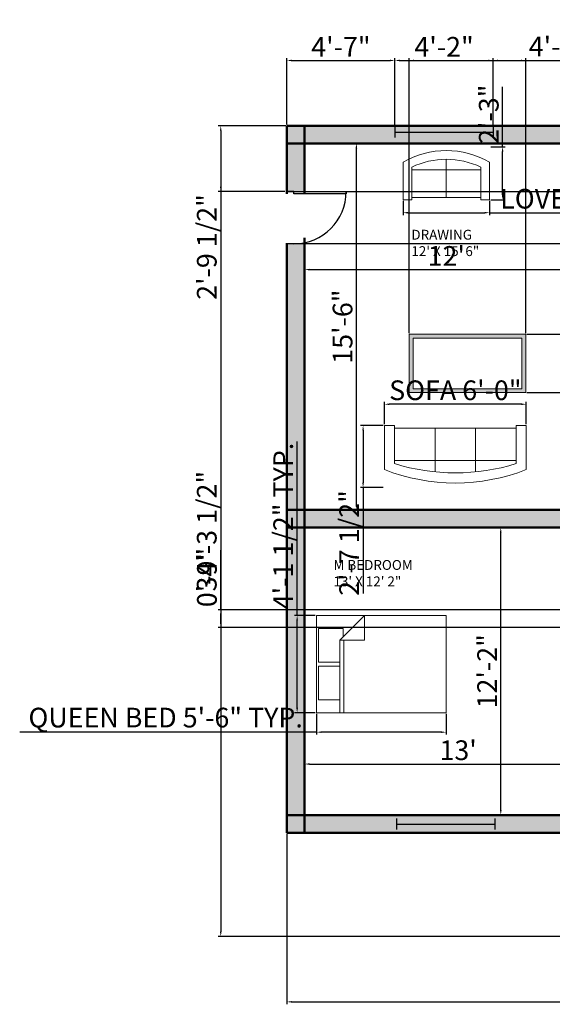
# Model space of a CAD drawing. Units: millimetres. Extents: x 2208 to 3043, y 878 to 1386.
# Tile 1 of 4: x 2208 to 2479, y 886 to 1386. Entities that reach past the tile are written whole.
import ezdxf

# ---------------------------------------------------------------- set-up
doc = ezdxf.new("R2010")
doc.units = ezdxf.units.MM
for name, color, linetype, lineweight in [('A-ANNO-DIMS', 50, 'Continuous', 13), ('A-AREA-IDEN', 90, 'Continuous', 25), ('A-WALL-PATT', 6, 'Continuous', 13), ('doors', 30, 'Continuous', 25), ('furniture', 140, 'Continuous', 18), ('walls', 200, 'Continuous', 50), ('windows', 10, 'Continuous', 25)]:
    doc.layers.add(name, color=color, linetype=linetype, lineweight=lineweight)
doc.layers.add('A-FURN-PATT', color=152, linetype='Continuous', lineweight=13, true_color=0x2776bb)
doc.styles.get("Standard").update_dxf_attribs({"font": 'arial.ttf'})
doc.dimstyles.new('ISO-25', dxfattribs={"dimtxt": 10, "dimasz": 2.5, "dimexe": 1.25, "dimexo": 0.625, "dimtad": 1, "dimdec": 0, "dimlunit": 3, "dimtxsty": 'Standard', "dimcen": 2.5, "dimadec": 0, "dimazin": 0, "dimtfac": 1, "dimtdec": 0, "dimtmove": 0, "dimatfit": 3, "dimfxl": 1, "dimarcsym": 0})

# ---------------------------------------------------------------- blocks, each defined once
blk = doc.blocks.new('*U2')
for p, q in [((0, 0), (0, -6)), ((40, 0), (40, -6))]:
    blk.add_line(p, q)
blk.add_lwpolyline([(0, 0), (0, 40), (1.75, 40), (1.75, 0)], close=True)
blk.add_arc((0, 0), 40, 0, 90)
blk = doc.blocks.new('*U4')
for p, q in [((0, 4), (0, 0)), ((36, 4), (36, 0)), ((0, 2), (36, 2))]:
    blk.add_line(p, q)
blk = doc.blocks.new('Bed - Queen')
for p, q in [((0, -80.00003), (0, 0)), ((0, 0), (59.99999, 0)), ((59.99999, 0), (59.99999, -80.00003)), ((7.99999, -1.2), (28.79998, -1.2)), ((7.99999, -14.4), (7.99999, -1.2)), ((28.79998, -1.2), (28.79998, -14.4)), ((31.19999, -1.2), (51.99999, -1.2)), ((31.19999, -14.4), (31.19999, -1.2)), ((51.99999, -1.2), (51.99999, -16.4)), ((0, -14.4), (44.8, -14.4)), ((44.8, -16.8), (0, -16.8)), ((59.99999, -29.6), (44.8, -14.4)), ((44.8, -14.4), (44.8, -29.6)), ((51.99999, -16.4), (46.79936, -16.4)), ((44.8, -29.6), (59.99999, -29.6)), ((59.99999, -80.00003), (0, -80.00003))]:
    blk.add_line(p, q)
blk = doc.blocks.new('Sofa - Roundback 7 ft.')
for p, q in [((-36.000027, -34), (-36.000027, -11.4696)), ((-12.00002, -32.4421), (-12.00003, -6.5971)), ((11.99997, -32.4421), (11.99998, -6.5971)), ((35.99998, -34), (35.99998, -11.4696)), ((-35.999844, -13.3819), (35.9998, -13.3819)), ((-36.000027, -32.4421), (35.99998, -32.4421))]:
    blk.add_line(p, q)
for points in [[(-36.000027, -34), (-42.000027, -34), (-42.000027, -8)], [(41.99998, -8), (41.99998, -34), (35.99998, -34)]]:
    blk.add_lwpolyline(points)
for centre, radius, start, end in [((0, -114.25), 114.25, 68.43141, 111.5686), ((-0.00001, -127.1968), 121.1968, 72.72033, 107.2797)]:
    blk.add_arc(centre, radius, start, end)
blk = doc.blocks.new('Sofa - Roundback Loveseat 5 ft.')
for p, q in [((0, -32.44198), (0, -5.99998)), ((-24, -33.99998), (-24, -11.46958)), ((-23.9998, -13.38178), (23.99986, -13.38178)), ((24.00004, -33.99998), (24.00004, -11.46958)), ((-24, -32.44198), (24.00004, -32.44198))]:
    blk.add_line(p, q)
for points in [[(-24, -33.99998), (-30, -33.99998), (-30, -7.99998)], [(30.00004, -7.99998), (30.00004, -33.99998), (24.00004, -33.99998)]]:
    blk.add_lwpolyline(points)
for centre, radius, start, end in [((0, -60.24998), 60.24998, 60.13715, 119.8628), ((0, -61.38438), 55.38444, 64.32083, 115.6792)]:
    blk.add_arc(centre, radius, start, end)
blk = doc.blocks.new('*D15')
at = {"layer": 'A-ANNO-DIMS', "color": 0, "lineweight": -2, "transparency": 16777216}
for p, q in [((2352.98, 1251.32), (2352.98, 1260.64)), ((2496.98, 1251.32), (2496.98, 1260.64)), ((2355.48, 1259.39), (2494.48, 1259.39))]:
    blk.add_line(p, q, dxfattribs=at)
at = {"layer": 'A-ANNO-DIMS', "color": 0, "transparency": 16777216}
for points in [[(2355.48, 1259.81), (2355.48, 1258.97), (2352.98, 1259.39)], [(2494.48, 1259.81), (2494.48, 1258.97), (2496.98, 1259.39)]]:
    blk.add_solid(points, dxfattribs=at)
at = {"layer": 'Defpoints', "color": 0, "transparency": 16777216}
for p in [(2496.98, 1259.39), (2352.98, 1250.7), (2496.98, 1250.7)]:
    blk.add_point(p, dxfattribs=at)
at = {"layer": 'A-ANNO-DIMS', "color": 0, "transparency": 16777216, "insert": (2424.98, 1265.03), "char_height": 10, "attachment_point": 5}
blk.add_mtext("12'", dxfattribs=at)
blk = doc.blocks.new('*D16')
at = {"layer": 'A-ANNO-DIMS', "color": 0, "lineweight": -2, "transparency": 16777216}
for p, q in [((2376.11, 1323.44), (2380.54, 1323.44)), ((2379.29, 1139.94), (2379.29, 1320.94)), ((2372.31, 1137.44), (2380.54, 1137.44))]:
    blk.add_line(p, q, dxfattribs=at)
at = {"layer": 'A-ANNO-DIMS', "color": 0, "transparency": 16777216}
for points in [[(2378.87, 1320.94), (2379.71, 1320.94), (2379.29, 1323.44)], [(2378.87, 1139.94), (2379.71, 1139.94), (2379.29, 1137.44)]]:
    blk.add_solid(points, dxfattribs=at)
at = {"layer": 'Defpoints', "color": 0, "transparency": 16777216}
for p in [(2375.49, 1323.44), (2379.29, 1323.44), (2371.69, 1137.44)]:
    blk.add_point(p, dxfattribs=at)
at = {"layer": 'A-ANNO-DIMS', "color": 0, "transparency": 16777216, "insert": (2373.56, 1230.44), "char_height": 10, "attachment_point": 5, "rotation": 90}
blk.add_mtext('15\'-6"', dxfattribs=at)
blk = doc.blocks.new('*D21')
at = {"layer": 'A-ANNO-DIMS', "color": 0, "lineweight": -2, "transparency": 16777216}
for p, q in [((2470.86, 1128.44), (2451.4, 1128.44)), ((2452.65, 984.94), (2452.65, 1125.94)), ((2470.86, 982.44), (2451.4, 982.44))]:
    blk.add_line(p, q, dxfattribs=at)
at = {"layer": 'A-ANNO-DIMS', "color": 0, "transparency": 16777216}
for points in [[(2452.23, 1125.94), (2453.07, 1125.94), (2452.65, 1128.44)], [(2452.23, 984.94), (2453.07, 984.94), (2452.65, 982.44)]]:
    blk.add_solid(points, dxfattribs=at)
at = {"layer": 'Defpoints', "color": 0, "transparency": 16777216}
for p in [(2452.65, 1128.44), (2471.48, 1128.44), (2471.48, 982.44)]:
    blk.add_point(p, dxfattribs=at)
at = {"layer": 'A-ANNO-DIMS', "color": 0, "transparency": 16777216, "insert": (2447, 1055.44), "char_height": 10, "attachment_point": 5, "rotation": 90}
blk.add_mtext('12\'-2"', dxfattribs=at)
blk = doc.blocks.new('*D22')
at = {"layer": 'A-ANNO-DIMS', "color": 0, "lineweight": -2, "transparency": 16777216}
for p, q in [((2352.98, 996.86), (2352.98, 1009.56)), ((2355.48, 1008.31), (2506.48, 1008.31)), ((2508.98, 996.86), (2508.98, 1009.56))]:
    blk.add_line(p, q, dxfattribs=at)
at = {"layer": 'A-ANNO-DIMS', "color": 0, "transparency": 16777216}
for points in [[(2355.48, 1008.73), (2355.48, 1007.9), (2352.98, 1008.31)], [(2506.48, 1008.73), (2506.48, 1007.9), (2508.98, 1008.31)]]:
    blk.add_solid(points, dxfattribs=at)
at = {"layer": 'Defpoints', "color": 0, "transparency": 16777216}
for p in [(2508.98, 1008.31), (2352.98, 996.23), (2508.98, 996.23)]:
    blk.add_point(p, dxfattribs=at)
at = {"layer": 'A-ANNO-DIMS', "color": 0, "transparency": 16777216, "insert": (2430.98, 1014.05), "char_height": 10, "attachment_point": 5}
blk.add_mtext("13'", dxfattribs=at)
blk = doc.blocks.new('*D36')
at = {"layer": 'A-ANNO-DIMS', "color": 0, "lineweight": -2, "transparency": 16777216}
for p, q in [((2359.06, 1033.76), (2359.06, 1023.26)), ((2424.9, 1033.76), (2424.9, 1023.26)), ((2359.06, 1024.51), (2208.21, 1024.51)), ((2422.4, 1024.51), (2361.56, 1024.51))]:
    blk.add_line(p, q, dxfattribs=at)
at = {"layer": 'A-ANNO-DIMS', "color": 0, "transparency": 16777216}
for points in [[(2361.56, 1024.92), (2361.56, 1024.09), (2359.06, 1024.51)], [(2422.4, 1024.92), (2422.4, 1024.09), (2424.9, 1024.51)]]:
    blk.add_solid(points, dxfattribs=at)
at = {"layer": 'Defpoints', "color": 0, "transparency": 16777216}
for p in [(2359.06, 1034.38), (2424.9, 1034.38), (2359.06, 1024.51)]:
    blk.add_point(p, dxfattribs=at)
at = {"layer": 'A-ANNO-DIMS', "color": 0, "transparency": 16777216, "insert": (2282.38, 1030.61), "char_height": 10, "attachment_point": 5}
blk.add_mtext('QUEEN BED 5\'-6" TYP.', dxfattribs=at)
blk = doc.blocks.new('*D37')
at = {"layer": 'A-ANNO-DIMS', "color": 0, "lineweight": -2, "transparency": 16777216}
for p, q in [((2349.18, 1083.76), (2349.18, 1172.17)), ((2358.43, 1083.76), (2347.93, 1083.76)), ((2349.18, 1036.88), (2349.18, 1081.26)), ((2358.43, 1034.38), (2347.93, 1034.38))]:
    blk.add_line(p, q, dxfattribs=at)
at = {"layer": 'A-ANNO-DIMS', "color": 0, "transparency": 16777216}
for points in [[(2348.77, 1081.26), (2349.6, 1081.26), (2349.18, 1083.76)], [(2348.77, 1036.88), (2349.6, 1036.88), (2349.18, 1034.38)]]:
    blk.add_solid(points, dxfattribs=at)
at = {"layer": 'Defpoints', "color": 0, "transparency": 16777216}
for p in [(2349.18, 1083.76), (2359.06, 1083.76), (2359.06, 1034.38)]:
    blk.add_point(p, dxfattribs=at)
at = {"layer": 'A-ANNO-DIMS', "color": 0, "transparency": 16777216, "insert": (2343.39, 1129.22), "char_height": 10, "attachment_point": 5, "rotation": 90}
blk.add_mtext('4\'-1 1/2" TYP.', dxfattribs=at)
blk = doc.blocks.new('*D42')
at = {"layer": 'A-ANNO-DIMS', "color": 0, "lineweight": -2, "transparency": 16777216}
for p, q in [((2393.52, 1180.83), (2393.52, 1192.27)), ((2463.14, 1191.02), (2396.02, 1191.02)), ((2465.64, 1180.83), (2465.64, 1192.27))]:
    blk.add_line(p, q, dxfattribs=at)
at = {"layer": 'A-ANNO-DIMS', "color": 0, "transparency": 16777216}
for points in [[(2396.02, 1191.44), (2396.02, 1190.61), (2393.52, 1191.02)], [(2463.14, 1191.44), (2463.14, 1190.61), (2465.64, 1191.02)]]:
    blk.add_solid(points, dxfattribs=at)
at = {"layer": 'Defpoints', "color": 0, "transparency": 16777216}
for p in [(2393.52, 1191.02), (2393.52, 1180.2), (2465.64, 1180.2)]:
    blk.add_point(p, dxfattribs=at)
at = {"layer": 'A-ANNO-DIMS', "color": 0, "transparency": 16777216, "insert": (2429.58, 1196.82), "char_height": 10, "attachment_point": 5}
blk.add_mtext('SOFA 6\'-0"', dxfattribs=at)
blk = doc.blocks.new('*D43')
at = {"layer": 'A-ANNO-DIMS', "color": 0, "lineweight": -2, "transparency": 16777216}
for p, q in [((2392.89, 1180.2), (2381.45, 1180.2)), ((2382.7, 1177.7), (2382.7, 1151.22)), ((2392.89, 1148.72), (2381.45, 1148.72)), ((2382.7, 1148.72), (2382.7, 1094.92))]:
    blk.add_line(p, q, dxfattribs=at)
at = {"layer": 'A-ANNO-DIMS', "color": 0, "transparency": 16777216}
for points in [[(2382.29, 1177.7), (2383.12, 1177.7), (2382.7, 1180.2)], [(2382.29, 1151.22), (2383.12, 1151.22), (2382.7, 1148.72)]]:
    blk.add_solid(points, dxfattribs=at)
at = {"layer": 'Defpoints', "color": 0, "transparency": 16777216}
for p in [(2393.52, 1180.2), (2382.7, 1148.72), (2393.52, 1148.72)]:
    blk.add_point(p, dxfattribs=at)
at = {"layer": 'A-ANNO-DIMS', "color": 0, "transparency": 16777216, "insert": (2376.91, 1120.57), "char_height": 10, "attachment_point": 5, "rotation": 90}
blk.add_mtext('2\'-7 1/2"', dxfattribs=at)
blk = doc.blocks.new('*D44')
at = {"layer": 'A-ANNO-DIMS', "color": 0, "lineweight": -2, "transparency": 16777216}
for p, q in [((2402.99, 1294.26), (2402.99, 1287.04)), ((2446.98, 1294.26), (2446.98, 1287.04)), ((2405.49, 1288.29), (2444.48, 1288.29)), ((2446.98, 1288.29), (2554.51, 1288.29))]:
    blk.add_line(p, q, dxfattribs=at)
at = {"layer": 'A-ANNO-DIMS', "color": 0, "transparency": 16777216}
for points in [[(2405.49, 1288.7), (2405.49, 1287.87), (2402.99, 1288.29)], [(2444.48, 1288.7), (2444.48, 1287.87), (2446.98, 1288.29)]]:
    blk.add_solid(points, dxfattribs=at)
at = {"layer": 'Defpoints', "color": 0, "transparency": 16777216}
for p in [(2402.99, 1294.89), (2446.98, 1294.89), (2446.98, 1288.29)]:
    blk.add_point(p, dxfattribs=at)
at = {"layer": 'A-ANNO-DIMS', "color": 0, "transparency": 16777216, "insert": (2502, 1294.09), "char_height": 10, "attachment_point": 5}
blk.add_mtext('LOVESEAT 3\'-8"', dxfattribs=at)
blk = doc.blocks.new('*D45')
at = {"layer": 'A-ANNO-DIMS', "color": 0, "lineweight": -2, "transparency": 16777216}
for p, q in [((2453.58, 1321.77), (2453.58, 1352.28)), ((2447.61, 1321.77), (2454.83, 1321.77)), ((2453.58, 1297.39), (2453.58, 1319.27)), ((2447.61, 1294.89), (2454.83, 1294.89))]:
    blk.add_line(p, q, dxfattribs=at)
at = {"layer": 'A-ANNO-DIMS', "color": 0, "transparency": 16777216}
for points in [[(2453.17, 1319.27), (2454, 1319.27), (2453.58, 1321.77)], [(2453.17, 1297.39), (2454, 1297.39), (2453.58, 1294.89)]]:
    blk.add_solid(points, dxfattribs=at)
at = {"layer": 'Defpoints', "color": 0, "transparency": 16777216}
for p in [(2446.98, 1321.77), (2453.58, 1321.77), (2446.98, 1294.89)]:
    blk.add_point(p, dxfattribs=at)
at = {"layer": 'A-ANNO-DIMS', "color": 0, "transparency": 16777216, "insert": (2447.85, 1338.28), "char_height": 10, "attachment_point": 5, "rotation": 90}
blk.add_mtext('2\'-3"', dxfattribs=at)
blk = doc.blocks.new('*D46')
at = {"layer": 'A-ANNO-DIMS', "color": 0, "lineweight": -2, "transparency": 16777216}
for p, q in [((3001.16, 1077), (3001.16, 886.32)), ((2343.98, 972.81), (2343.98, 886.32)), ((2346.48, 887.57), (2998.66, 887.57))]:
    blk.add_line(p, q, dxfattribs=at)
at = {"layer": 'A-ANNO-DIMS', "color": 0, "transparency": 16777216}
for points in [[(2346.48, 887.99), (2346.48, 887.16), (2343.98, 887.57)], [(2998.66, 887.99), (2998.66, 887.16), (3001.16, 887.57)]]:
    blk.add_solid(points, dxfattribs=at)
at = {"layer": 'Defpoints', "color": 0, "transparency": 16777216}
for p in [(3001.16, 1077.62), (2343.98, 973.44), (3001.16, 887.57)]:
    blk.add_point(p, dxfattribs=at)
at = {"layer": 'A-ANNO-DIMS', "color": 0, "transparency": 16777216, "insert": (2672.57, 893.3), "char_height": 10, "attachment_point": 5}
blk.add_mtext('54\'-9"', dxfattribs=at)
blk = doc.blocks.new('*D47')
at = {"layer": 'A-ANNO-DIMS', "color": 0, "lineweight": -2, "transparency": 16777216}
for p, q in [((2343.36, 1332.44), (2309.12, 1332.44)), ((2310.37, 1329.94), (2310.37, 923.22)), ((2589.36, 920.72), (2309.12, 920.72))]:
    blk.add_line(p, q, dxfattribs=at)
at = {"layer": 'A-ANNO-DIMS', "color": 0, "transparency": 16777216}
for points in [[(2309.95, 1329.94), (2310.79, 1329.94), (2310.37, 1332.44)], [(2309.95, 923.22), (2310.79, 923.22), (2310.37, 920.72)]]:
    blk.add_solid(points, dxfattribs=at)
at = {"layer": 'Defpoints', "color": 0, "transparency": 16777216}
for p in [(2343.98, 1332.44), (2310.37, 920.72), (2589.98, 920.72)]:
    blk.add_point(p, dxfattribs=at)
at = {"layer": 'A-ANNO-DIMS', "color": 0, "transparency": 16777216, "insert": (2304.57, 1126.58), "char_height": 10, "attachment_point": 5, "rotation": 90}
blk.add_mtext('34\'-3 1/2"', dxfattribs=at)
blk = doc.blocks.new('*D51')
at = {"layer": 'A-ANNO-DIMS', "color": 0, "lineweight": -2, "transparency": 16777216}
for p, q in [((2344.15, 1299.03), (3035.56, 1299.03)), ((3034.31, 1296.53), (3034.31, 1275.14)), ((2344.61, 1272.64), (3035.56, 1272.64)), ((3034.31, 1272.64), (3034.31, 1218.83))]:
    blk.add_line(p, q, dxfattribs=at)
at = {"layer": 'A-ANNO-DIMS', "color": 0, "transparency": 16777216}
for points in [[(3033.9, 1296.53), (3034.73, 1296.53), (3034.31, 1299.03)], [(3033.9, 1275.14), (3034.73, 1275.14), (3034.31, 1272.64)]]:
    blk.add_solid(points, dxfattribs=at)
at = {"layer": 'Defpoints', "color": 0, "transparency": 16777216}
for p in [(2343.52, 1299.03), (2343.98, 1272.64), (3034.31, 1272.64)]:
    blk.add_point(p, dxfattribs=at)
at = {"layer": 'A-ANNO-DIMS', "color": 0, "transparency": 16777216, "insert": (3028.52, 1244.49), "char_height": 10, "attachment_point": 5, "rotation": 90}
blk.add_mtext('2\'-2 1/2"', dxfattribs=at)
blk = doc.blocks.new('*D52')
at = {"layer": 'A-ANNO-DIMS', "color": 0, "lineweight": -2, "transparency": 16777216}
for p, q in [((2343.36, 1332.44), (2309.12, 1332.44)), ((2310.37, 1329.94), (2310.37, 1301.53)), ((2342.9, 1299.03), (2309.12, 1299.03)), ((2310.37, 1299.03), (2310.37, 1245.23))]:
    blk.add_line(p, q, dxfattribs=at)
at = {"layer": 'A-ANNO-DIMS', "color": 0, "transparency": 16777216}
for points in [[(2309.95, 1329.94), (2310.79, 1329.94), (2310.37, 1332.44)], [(2309.95, 1301.53), (2310.79, 1301.53), (2310.37, 1299.03)]]:
    blk.add_solid(points, dxfattribs=at)
at = {"layer": 'Defpoints', "color": 0, "transparency": 16777216}
for p in [(2343.98, 1332.44), (2310.37, 1299.03), (2343.52, 1299.03)]:
    blk.add_point(p, dxfattribs=at)
at = {"layer": 'A-ANNO-DIMS', "color": 0, "transparency": 16777216, "insert": (2304.57, 1270.88), "char_height": 10, "attachment_point": 5, "rotation": 90}
blk.add_mtext('2\'-9 1/2"', dxfattribs=at)
blk = doc.blocks.new('*D53')
at = {"layer": 'A-ANNO-DIMS', "color": 0, "lineweight": -2, "transparency": 16777216}
for p, q in [((2343.98, 1333.06), (2343.98, 1366.84)), ((2346.48, 1365.59), (2396.36, 1365.59)), ((2398.86, 1332.56), (2398.86, 1366.84))]:
    blk.add_line(p, q, dxfattribs=at)
at = {"layer": 'A-ANNO-DIMS', "color": 0, "transparency": 16777216}
for points in [[(2346.48, 1366), (2346.48, 1365.17), (2343.98, 1365.59)], [(2396.36, 1366), (2396.36, 1365.17), (2398.86, 1365.59)]]:
    blk.add_solid(points, dxfattribs=at)
at = {"layer": 'Defpoints', "color": 0, "transparency": 16777216}
for p in [(2398.86, 1365.59), (2343.98, 1332.44), (2398.86, 1331.94)]:
    blk.add_point(p, dxfattribs=at)
at = {"layer": 'A-ANNO-DIMS', "color": 0, "transparency": 16777216, "insert": (2371.42, 1371.21), "char_height": 10, "attachment_point": 5}
blk.add_mtext('4\'-7"', dxfattribs=at)
blk = doc.blocks.new('*D54')
at = {"layer": 'A-ANNO-DIMS', "color": 0, "lineweight": -2, "transparency": 16777216}
for p, q in [((2398.86, 1332.56), (2398.86, 1366.84)), ((2401.36, 1365.59), (2446.31, 1365.59)), ((2448.81, 1332.56), (2448.81, 1366.84))]:
    blk.add_line(p, q, dxfattribs=at)
at = {"layer": 'A-ANNO-DIMS', "color": 0, "transparency": 16777216}
for points in [[(2401.36, 1366), (2401.36, 1365.17), (2398.86, 1365.59)], [(2446.31, 1366), (2446.31, 1365.17), (2448.81, 1365.59)]]:
    blk.add_solid(points, dxfattribs=at)
at = {"layer": 'Defpoints', "color": 0, "transparency": 16777216}
for p in [(2448.81, 1365.59), (2398.86, 1331.94), (2448.81, 1331.94)]:
    blk.add_point(p, dxfattribs=at)
at = {"layer": 'A-ANNO-DIMS', "color": 0, "transparency": 16777216, "insert": (2423.84, 1371.23), "char_height": 10, "attachment_point": 5}
blk.add_mtext('4\'-2"', dxfattribs=at)
blk = doc.blocks.new('*D55')
at = {"layer": 'A-ANNO-DIMS', "color": 0, "lineweight": -2, "transparency": 16777216}
for p, q in [((2448.81, 1332.56), (2448.81, 1366.84)), ((2451.31, 1365.59), (2543.52, 1365.59)), ((2546.02, 1331.5), (2546.02, 1366.84))]:
    blk.add_line(p, q, dxfattribs=at)
at = {"layer": 'A-ANNO-DIMS', "color": 0, "transparency": 16777216}
for points in [[(2451.31, 1366), (2451.31, 1365.17), (2448.81, 1365.59)], [(2543.52, 1366), (2543.52, 1365.17), (2546.02, 1365.59)]]:
    blk.add_solid(points, dxfattribs=at)
at = {"layer": 'Defpoints', "color": 0, "transparency": 16777216}
for p in [(2546.02, 1365.59), (2448.81, 1331.94), (2546.02, 1330.88)]:
    blk.add_point(p, dxfattribs=at)
at = {"layer": 'A-ANNO-DIMS', "color": 0, "transparency": 16777216, "insert": (2497.42, 1371.32), "char_height": 10, "attachment_point": 5}
blk.add_mtext('8\'-1"', dxfattribs=at)
blk = doc.blocks.new('*D62')
at = {"layer": 'A-ANNO-DIMS', "color": 0, "lineweight": -2, "transparency": 16777216}
for p, q in [((2310.37, 1086.62), (2310.37, 1116.95)), ((3000.54, 1086.62), (2309.12, 1086.62)), ((2310.37, 1080.12), (2310.37, 1084.12)), ((3000.54, 1077.62), (2309.12, 1077.62))]:
    blk.add_line(p, q, dxfattribs=at)
at = {"layer": 'A-ANNO-DIMS', "color": 0, "transparency": 16777216}
for points in [[(2309.95, 1084.12), (2310.79, 1084.12), (2310.37, 1086.62)], [(2309.95, 1080.12), (2310.79, 1080.12), (2310.37, 1077.62)]]:
    blk.add_solid(points, dxfattribs=at)
at = {"layer": 'Defpoints', "color": 0, "transparency": 16777216}
for p in [(2310.37, 1086.62), (3001.16, 1086.62), (3001.16, 1077.62)]:
    blk.add_point(p, dxfattribs=at)
at = {"layer": 'A-ANNO-DIMS', "color": 0, "transparency": 16777216, "insert": (2304.64, 1103.04), "char_height": 10, "attachment_point": 5, "rotation": 90}
blk.add_mtext('0\'-9"', dxfattribs=at)
blk = doc.blocks.new('*D63')
at = {"layer": 'A-ANNO-DIMS', "color": 0, "lineweight": -2, "transparency": 16777216}
for p, q in [((2406.08, 1227.17), (2406.08, 1366.84)), ((2408.58, 1365.59), (2462.85, 1365.59)), ((2465.35, 1227.17), (2465.35, 1366.84)), ((2465.35, 1365.59), (2527.15, 1365.59))]:
    blk.add_line(p, q, dxfattribs=at)
at = {"layer": 'A-ANNO-DIMS', "color": 0, "transparency": 16777216}
for points in [[(2408.58, 1366), (2408.58, 1365.17), (2406.08, 1365.59)], [(2462.85, 1366), (2462.85, 1365.17), (2465.35, 1365.59)]]:
    blk.add_solid(points, dxfattribs=at)
at = {"layer": 'Defpoints', "color": 0, "transparency": 16777216}
for p in [(2465.35, 1365.59), (2406.08, 1226.55), (2465.35, 1226.55)]:
    blk.add_point(p, dxfattribs=at)
at = {"layer": 'A-ANNO-DIMS', "color": 0, "transparency": 16777216, "insert": (2497.5, 1371.38), "char_height": 10, "attachment_point": 5}
blk.add_mtext('4\'-11 1/2"', dxfattribs=at)
blk = doc.blocks.new('*D64')
at = {"layer": 'A-ANNO-DIMS', "color": 0, "lineweight": -2, "transparency": 16777216}
for p, q in [((3034.31, 1226.55), (3034.31, 1280.35)), ((2465.97, 1226.55), (3035.56, 1226.55)), ((3034.31, 1199.41), (3034.31, 1224.05)), ((2465.97, 1196.91), (3035.56, 1196.91))]:
    blk.add_line(p, q, dxfattribs=at)
at = {"layer": 'A-ANNO-DIMS', "color": 0, "transparency": 16777216}
for points in [[(3033.9, 1224.05), (3034.73, 1224.05), (3034.31, 1226.55)], [(3033.9, 1199.41), (3034.73, 1199.41), (3034.31, 1196.91)]]:
    blk.add_solid(points, dxfattribs=at)
at = {"layer": 'Defpoints', "color": 0, "transparency": 16777216}
for p in [(2465.35, 1226.55), (3034.31, 1226.55), (2465.35, 1196.91)]:
    blk.add_point(p, dxfattribs=at)
at = {"layer": 'A-ANNO-DIMS', "color": 0, "transparency": 16777216, "insert": (3028.52, 1254.7), "char_height": 10, "attachment_point": 5, "rotation": 90}
blk.add_mtext('2\'-5 1/2"', dxfattribs=at)

msp = doc.modelspace()

# ---------------------------------------------------------------- hatches: boundary and pattern name
at = {"layer": 'A-FURN-PATT'}
h = msp.add_hatch(color=256, dxfattribs=at)
h.dxf.hatch_style = 1
h.paths.add_polyline_path([(2408.08, 1224.55), (2408.08, 1198.91), (2463.35, 1198.91), (2463.35, 1224.55)], flags=0)
h.paths.add_polyline_path([(2465.35, 1226.55), (2406.08, 1226.55), (2406.08, 1196.91), (2465.35, 1196.91)])
h.paths.add_polyline_path([(2463.35, 1224.55), (2463.35, 1198.91), (2408.08, 1198.91), (2408.08, 1224.55)], flags=16)
at = {"layer": 'A-WALL-PATT'}
h = msp.add_hatch(color=256, dxfattribs=at)
h.dxf.hatch_style = 1
h.paths.add_polyline_path([(2352.98, 1273, -0.051847), (2347.51, 1272.43), (2343.98, 1272.43), (2343.98, 1137.44), (2352.98, 1137.44)])
h.paths.add_polyline_path([(2352.98, 1323.44), (2343.98, 1323.44), (2343.98, 1299.03), (2347.51, 1299.03), (2352.98, 1299.03)])
h.paths.add_polyline_path([(2352.98, 1332.44), (2343.98, 1332.44), (2343.98, 1323.44), (2352.98, 1323.44)])
h.paths.add_polyline_path([(2496.98, 1332.44), (2352.98, 1332.44), (2352.98, 1323.44), (2496.98, 1323.44)])
h.paths.add_polyline_path([(2505.98, 1323.44), (2496.98, 1323.44), (2496.98, 1191.44), (2505.98, 1191.44)])
h.paths.add_polyline_path([(2505.98, 1332.44), (2496.98, 1332.44), (2496.98, 1323.44), (2505.98, 1323.44)])
h.paths.add_polyline_path([(2505.98, 1182.44), (2496.98, 1182.44), (2496.98, 1137.44), (2505.98, 1137.44)])
h.paths.add_polyline_path([(2505.98, 1191.44), (2496.98, 1191.44), (2496.98, 1182.44), (2505.98, 1182.44)])
h.paths.add_polyline_path([(2621.06, 1191.44), (2505.98, 1191.44), (2505.98, 1182.44), (2619.92, 1182.44), (2619.92, 1183.73, -0.073589)])
h.paths.add_polyline_path([(2496.98, 1137.44), (2352.98, 1137.44), (2352.98, 1128.44), (2496.98, 1128.44)])
h.paths.add_polyline_path([(2352.98, 1137.44), (2343.98, 1137.44), (2343.98, 1128.44), (2352.98, 1128.44)])
h.paths.add_polyline_path([(2352.98, 1128.44), (2343.98, 1128.44), (2343.98, 982.44), (2352.98, 982.44)])
h.paths.add_polyline_path([(2517.98, 1137.44), (2508.98, 1137.44), (2508.98, 1128.44), (2517.98, 1128.44)])
h.paths.add_polyline_path([(2505.98, 1137.44), (2496.98, 1137.44), (2496.98, 1128.44), (2505.98, 1128.44)])
h.paths.add_polyline_path([(2658.98, 1224.44), (2649.98, 1224.44), (2649.98, 1191.44), (2658.98, 1191.44)])
h.paths.add_polyline_path([(2658.98, 1323.44), (2649.98, 1323.44), (2649.98, 1233.44), (2658.98, 1233.44)])
h.paths.add_polyline_path([(2658.98, 1233.44), (2649.98, 1233.44), (2649.98, 1224.44), (2658.98, 1224.44)])
h.paths.add_polyline_path([(2730.98, 1233.44), (2658.98, 1233.44), (2658.98, 1224.44), (2730.98, 1224.44)])
h.paths.add_polyline_path([(2739.98, 1323.44), (2730.98, 1323.44), (2730.98, 1233.44), (2739.98, 1233.44)])
h.paths.add_polyline_path([(2739.98, 1224.44), (2730.98, 1224.44), (2730.98, 1191.44), (2739.98, 1191.44)])
h.paths.add_polyline_path([(2739.98, 1191.44), (2730.98, 1191.44), (2730.98, 1182.44), (2739.98, 1182.44)])
h.paths.add_polyline_path([(2739.98, 1182.44), (2730.98, 1182.44), (2730.98, 1171.44), (2739.98, 1171.44)])
h.paths.add_polyline_path([(2739.98, 972.44), (2730.98, 972.44), (2730.98, 929.72), (2602.15, 929.72), (2598.98, 929.72), (2598.98, 973.44), (2589.98, 973.44), (2589.98, 929.72), (2589.98, 920.72), (2730.98, 920.72), (2739.98, 920.72)])
h.paths.add_polyline_path([(2598.98, 1084.44), (2589.98, 1084.44), (2589.98, 982.44), (2598.98, 982.44)])
h.paths.add_polyline_path([(2598.98, 982.44), (2589.98, 982.44), (2589.98, 973.44), (2598.98, 973.44)])
h.paths.add_polyline_path([(2517.98, 973.44), (2508.98, 973.44), (2508.98, 944.53), (2517.98, 944.53)])
h.paths.add_polyline_path([(2517.98, 1044.76, -0.086498), (2508.98, 1043.19), (2508.98, 982.44), (2517.98, 982.44)])
h.paths.add_polyline_path([(2517.98, 982.44), (2508.98, 982.44), (2508.98, 973.44), (2517.98, 973.44)])
h.paths.add_polyline_path([(2352.98, 982.44), (2343.98, 982.44), (2343.98, 973.44), (2352.98, 973.44)])
h.paths.add_polyline_path([(2589.98, 1093.44), (2517.98, 1093.44), (2517.98, 1084.44), (2589.98, 1084.44)])
h.paths.add_polyline_path([(2517.98, 1093.44), (2508.98, 1093.44), (2508.98, 1084.44), (2517.98, 1084.44)])
h.paths.add_polyline_path([(2517.98, 1084.44), (2508.98, 1084.44), (2508.98, 1069.79), (2517.98, 1069.79)])
h.paths.add_polyline_path([(2517.98, 1100.83), (2517.21, 1100.83, -0.078775), (2508.98, 1102.14), (2508.98, 1093.44), (2517.98, 1093.44)])
h.paths.add_polyline_path([(2598.98, 1093.44), (2589.98, 1093.44), (2589.98, 1084.44), (2598.98, 1084.44)])
h.paths.add_polyline_path([(2802.98, 1122.44), (2730.98, 1122.44), (2730.98, 1113.44), (2802.98, 1113.44)])
h.paths.add_polyline_path([(2922.98, 1113.44), (2913.98, 1113.44), (2913.98, 981.44), (2922.98, 981.44)])
h.paths.add_polyline_path([(2856.98, 1069.77, -0.087206), (2847.98, 1067.81), (2847.98, 981.44), (2856.98, 981.44)])
h.paths.add_polyline_path([(2913.98, 981.44), (2856.98, 981.44), (2856.98, 972.44), (2913.98, 972.44)])
h.paths.add_polyline_path([(2856.98, 981.44), (2847.98, 981.44), (2847.98, 972.44), (2856.98, 972.44)])
h.paths.add_polyline_path([(2739.98, 995.72), (2739.98, 1004.72), (2730.98, 1004.72), (2730.98, 981.44), (2739.98, 981.44)])
h.paths.add_polyline_path([(2739.98, 981.44), (2730.98, 981.44), (2730.98, 972.44), (2739.98, 972.44)])
h.paths.add_polyline_path([(2922.98, 981.44), (2913.98, 981.44), (2913.98, 972.44), (2922.98, 972.44)])
h.paths.add_polyline_path([(3001.16, 1086.62), (2922.98, 1086.62), (2922.98, 1077.62), (3001.16, 1077.62)])
h.paths.add_polyline_path([(3001.16, 1191.44), (2922.98, 1191.44), (2922.98, 1182.44), (3001.16, 1182.44)])
h.paths.add_polyline_path([(2913.98, 1191.44), (2843.61, 1191.44), (2843.49, 1188.69, -0.05974), (2842.46, 1182.44), (2913.98, 1182.44)])
h.paths.add_polyline_path([(2922.98, 1191.44), (2913.98, 1191.44), (2913.98, 1182.44), (2922.98, 1182.44)])
h.paths.add_polyline_path([(2802.98, 1191.44), (2769.17, 1191.44, -0.079558), (2770.5, 1183.13), (2770.5, 1182.44), (2802.98, 1182.44)])
h.paths.add_polyline_path([(2811.98, 1191.44), (2802.98, 1191.44), (2802.98, 1182.44), (2811.98, 1182.44)])
h.paths.add_polyline_path([(2811.98, 1182.44), (2802.98, 1182.44), (2802.98, 1122.44), (2811.98, 1122.44)])
h.paths.add_polyline_path([(2811.98, 1122.44), (2802.98, 1122.44), (2802.98, 1113.44), (2811.98, 1113.44)])
h.paths.add_polyline_path([(2847.98, 1122.44), (2811.98, 1122.44), (2811.98, 1113.44), (2847.98, 1113.44)])
h.paths.add_polyline_path([(2856.98, 1122.44), (2847.98, 1122.44), (2847.98, 1113.44), (2856.98, 1113.44)])
h.paths.add_polyline_path([(2913.98, 1122.44), (2856.98, 1122.44), (2856.98, 1113.44), (2913.98, 1113.44)])
h.paths.add_polyline_path([(2922.98, 1122.44), (2913.98, 1122.44), (2913.98, 1113.44), (2922.98, 1113.44)])
h.paths.add_polyline_path([(2856.98, 1113.44), (2847.98, 1113.44), (2847.98, 1094.39), (2856.98, 1094.39)])
h.paths.add_polyline_path([(2922.98, 1323.44), (2913.98, 1323.44), (2913.98, 1191.44), (2922.98, 1191.44)])
h.paths.add_polyline_path([(2922.98, 1332.44), (2913.98, 1332.44), (2913.98, 1323.44), (2922.98, 1323.44)])
h.paths.add_polyline_path([(2913.98, 1332.44), (2739.98, 1332.44), (2739.98, 1323.44), (2913.98, 1323.44)])
h.paths.add_polyline_path([(2730.98, 1332.44), (2658.98, 1332.44), (2658.98, 1323.44), (2730.98, 1323.44)])
h.paths.add_polyline_path([(2649.98, 1332.44), (2505.98, 1332.44), (2505.98, 1323.44), (2649.98, 1323.44)])
h.paths.add_polyline_path([(2658.98, 1332.44), (2649.98, 1332.44), (2649.98, 1323.44), (2658.98, 1323.44)])
h.paths.add_polyline_path([(2739.98, 1332.44), (2730.98, 1332.44), (2730.98, 1323.44), (2739.98, 1323.44)])
h.paths.add_polyline_path([(2739.98, 1233.44), (2730.98, 1233.44), (2730.98, 1224.44), (2739.98, 1224.44)])
h.paths.add_polyline_path([(2658.98, 1191.44), (2649.98, 1191.44), (2649.98, 1182.44), (2658.98, 1182.44)])
h.paths.add_polyline_path([(2658.98, 1182.44), (2649.98, 1182.44), (2649.98, 1171.44), (2658.98, 1171.44)])
h.paths.add_polyline_path([(2508.98, 982.44), (2352.98, 982.44), (2352.98, 973.44), (2508.98, 973.44)])
h.paths.add_polyline_path([(2589.98, 982.44), (2517.98, 982.44), (2517.98, 973.44), (2589.98, 973.44)])
h.paths.add_polyline_path([(2730.98, 1004.72), (2598.98, 1004.72), (2598.98, 995.72), (2730.98, 995.72)])
h.paths.add_polyline_path([(2847.98, 981.44), (2739.98, 981.44), (2739.98, 972.44), (2847.98, 972.44)])

# ---------------------------------------------------------------- linework, layer by layer
at = {"layer": 'furniture'}
for p, q in [((2406.08, 1226.55), (2406.08, 1196.91)), ((2465.35, 1226.55), (2406.08, 1226.55)), ((2465.35, 1196.91), (2465.35, 1226.55)), ((2408.08, 1224.55), (2408.08, 1198.91)), ((2463.35, 1224.55), (2408.08, 1224.55)), ((2463.35, 1198.91), (2463.35, 1224.55)), ((2406.08, 1196.91), (2465.35, 1196.91)), ((2408.08, 1198.91), (2463.35, 1198.91))]:
    msp.add_line(p, q, dxfattribs=at)
at = {"layer": 'walls'}
for p, q in [((2343.98, 1332.44), (2343.98, 1297.87)), ((2343.98, 1332.44), (2922.98, 1332.44)), ((2352.98, 1332.44), (2352.98, 1297.87)), ((2343.98, 1323.44), (2922.98, 1323.44)), ((2352.98, 1275.45), (2352.98, 973.44)), ((2343.98, 1272.64), (2343.98, 973.44)), ((2343.98, 1137.44), (2517.98, 1137.44)), ((2343.98, 1128.44), (2517.98, 1128.44)), ((2343.98, 982.44), (2598.98, 982.44)), ((2343.98, 973.44), (2598.98, 973.44))]:
    msp.add_line(p, q, dxfattribs=at)

# ---------------------------------------------------------------- block references
at = {"layer": 'doors', "xscale": 0.6650461219051067, "yscale": 0.6650461219051067, "zscale": 0.6650461219051067, "rotation": 270}
msp.add_blockref('*U2', (2347.51, 1299.03), dxfattribs=at)
at = {"layer": 'furniture', "xscale": 0.7332754359168536, "yscale": 0.7332754359168536, "zscale": 0.7332754359168536}
msp.add_blockref('Sofa - Roundback Loveseat 5 ft.', (2424.98, 1319.82), dxfattribs=at)
at = {"layer": 'furniture'}
for name, p, xscale, yscale, zscale, rotation in [('Sofa - Roundback 7 ft.', (2429.58, 1151.01), 0.8585581732242188, 0.8585581732242188, 0.8585581732242188, 180), ('Bed - Queen', (2359.06, 1034.38), 0.8230212393777605, 0.8230212393777605, 0.8230212393777605, 90)]:
    msp.add_blockref(name, p, dxfattribs=dict(at, xscale=xscale, yscale=yscale, zscale=zscale, rotation=rotation))
at = {"layer": 'windows', "xscale": 1.38727767019332, "yscale": 1.38727767019332, "zscale": 1.38727767019332}
for p in [(2398.86, 1326.39), (2399.64, 975.09)]:
    msp.add_blockref('*U4', p, dxfattribs=at)

# ---------------------------------------------------------------- texts
at = {"layer": 'A-AREA-IDEN', "char_height": 5, "attachment_point": 1}
for s, width, insert in [('DRAWING \\P12\' X 15\' 6"', 44.034, (2407.24, 1279.61)), ('M BEDROOM\\P13\' X 12\' 2"', 66.6081, (2367.66, 1111.92))]:
    msp.add_mtext_dynamic_manual_height_columns(s, width=width, gutter_width=12.5, heights=[0], dxfattribs=dict(at, insert=insert))

# ---------------------------------------------------------------- dimensions: what is measured, and where the dimension line sits
at = {"layer": 'A-ANNO-DIMS'}
for base, p1, p2, override, picture, middle in [((2465.35, 1365.59), (2406.08, 1226.55), (2465.35, 1226.55), {"dimdec": 1, "dimlfac": 1, "dimrnd": 0, "dimzin": 1, "dimdsep": 46, "dimlunit": 4, "dimfrac": 2}, '*D63', (2497.5, 1371.38)), ((2398.86, 1365.59), (2343.98, 1332.44), (2398.86, 1331.94), {"dimdec": 1, "dimlfac": 1, "dimrnd": 0, "dimzin": 1, "dimdsep": 46, "dimlunit": 4, "dimfrac": 2}, '*D53', (2371.42, 1371.21)), ((2448.807, 1365.5855), (2398.865, 1331.936), (2448.807, 1331.936), {"dimdec": 1, "dimlfac": 1, "dimrnd": 0, "dimzin": 1, "dimdsep": 46, "dimlunit": 4, "dimfrac": 2}, '*D54', (2423.836, 1371.231)), ((2546.02, 1365.59), (2448.81, 1331.94), (2546.02, 1330.88), {"dimdec": 1, "dimlfac": 1, "dimrnd": 0, "dimzin": 1, "dimdsep": 46, "dimlunit": 4, "dimfrac": 2}, '*D55', (2497.42, 1371.32)), ((2496.98, 1259.39), (2352.98, 1250.7), (2496.98, 1250.7), {"dimclrd": 0, "dimclre": 0, "dimclrt": 0}, '*D15', (2424.98, 1265.03)), ((3001.16, 887.57), (2343.98, 973.44), (3001.16, 1077.62), {"dimdec": 1, "dimlfac": 1, "dimrnd": 0, "dimzin": 1, "dimdsep": 46, "dimlunit": 4, "dimfrac": 2}, '*D46', (2672.57, 893.3)), ((2508.98, 1008.31), (2352.98, 996.23), (2508.98, 996.23), {"dimclrd": 0, "dimclre": 0, "dimclrt": 0}, '*D22', (2430.98, 1014.05))]:
    dim = msp.add_linear_dim(base=base, p1=p1, p2=p2, dimstyle='ISO-25', override=override, dxfattribs=at)
    dim.commit()
    dim.dimension.update_dxf_attribs({"geometry": picture, "text_midpoint": middle})
for base, p1, p2, angle, override, picture, middle in [((2453.58, 1321.77), (2446.98, 1294.89), (2446.98, 1321.77), 90, {"dimdec": 1, "dimlfac": 1, "dimrnd": 0, "dimzin": 1, "dimdsep": 46, "dimlunit": 4, "dimfrac": 2}, '*D45', (2447.85, 1338.28)), ((2310.37, 920.72), (2343.98, 1332.44), (2589.98, 920.72), 90, {"dimdec": 1, "dimlfac": 1, "dimrnd": 0, "dimzin": 1, "dimdsep": 46, "dimlunit": 4, "dimfrac": 2}, '*D47', (2304.57, 1126.58)), ((2310.37, 1299.03), (2343.98, 1332.44), (2343.52, 1299.03), 90, {"dimdec": 1, "dimlfac": 1, "dimrnd": 0, "dimzin": 1, "dimdsep": 46, "dimlunit": 4, "dimfrac": 2}, '*D52', (2304.57, 1270.88)), ((2379.29, 1323.44), (2371.69, 1137.44), (2375.49, 1323.44), 90, {"dimclrd": 0, "dimclre": 0, "dimclrt": 0}, '*D16', (2373.56, 1230.44)), ((3034.31, 1272.64), (2343.52, 1299.03), (2343.98, 1272.64), 90, {"dimdec": 1, "dimlfac": 1, "dimrnd": 0, "dimzin": 1, "dimdsep": 46, "dimlunit": 4, "dimfrac": 2}, '*D51', (3028.52, 1244.49)), ((3034.31, 1226.55), (2465.35, 1196.91), (2465.35, 1226.55), 90, {"dimdec": 1, "dimlfac": 1, "dimrnd": 0, "dimzin": 1, "dimdsep": 46, "dimlunit": 4, "dimfrac": 2}, '*D64', (3028.52, 1254.7)), ((2382.7, 1148.72), (2393.52, 1180.2), (2393.52, 1148.72), 270, {"dimdec": 1, "dimlfac": 1, "dimrnd": 0, "dimzin": 1, "dimdsep": 46, "dimlunit": 4, "dimfrac": 2}, '*D43', (2376.91, 1120.57)), ((2452.65, 1128.44), (2471.48, 982.44), (2471.48, 1128.44), 90, {"dimclrd": 0, "dimclre": 0, "dimclrt": 0}, '*D21', (2447, 1055.44)), ((2310.37, 1086.62), (3001.16, 1077.62), (3001.16, 1086.62), 90, {"dimdec": 1, "dimlfac": 1, "dimrnd": 0, "dimzin": 1, "dimdsep": 46, "dimlunit": 4, "dimfrac": 2}, '*D62', (2304.64, 1103.04))]:
    dim = msp.add_linear_dim(base=base, p1=p1, p2=p2, angle=angle, dimstyle='ISO-25', override=override, dxfattribs=at)
    dim.commit()
    dim.dimension.update_dxf_attribs({"geometry": picture, "text_midpoint": middle})
dim = msp.add_linear_dim(base=(2446.98, 1288.29), p1=(2402.99, 1294.89), p2=(2446.98, 1294.89), text='LOVESEAT <>', dimstyle='ISO-25', override={"dimdec": 1, "dimlfac": 1, "dimrnd": 0, "dimzin": 1, "dimdsep": 46, "dimlunit": 4, "dimfrac": 2}, dxfattribs=at)
dim.commit()
dim.dimension.update_dxf_attribs({"geometry": '*D44', "text_midpoint": (2502, 1294.09)})
for base, p1, p2, angle, text, picture, middle in [((2393.52, 1191.02), (2465.64, 1180.2), (2393.52, 1180.2), 180, 'SOFA <>', '*D42', (2429.58, 1196.82)), ((2349.18, 1083.76), (2359.06, 1034.38), (2359.06, 1083.76), 90, '<> TYP.', '*D37', (2343.39, 1129.22)), ((2359.06, 1024.51), (2424.9, 1034.38), (2359.06, 1034.38), 180, 'QUEEN BED <> TYP.', '*D36', (2282.38, 1030.61))]:
    dim = msp.add_linear_dim(base=base, p1=p1, p2=p2, angle=angle, text=text, dimstyle='ISO-25', override={"dimdec": 1, "dimlfac": 1, "dimrnd": 0, "dimzin": 1, "dimdsep": 46, "dimlunit": 4, "dimfrac": 2}, dxfattribs=at)
    dim.commit()
    dim.dimension.update_dxf_attribs({"geometry": picture, "text_midpoint": middle})

doc.saveas('drawing.dxf')
